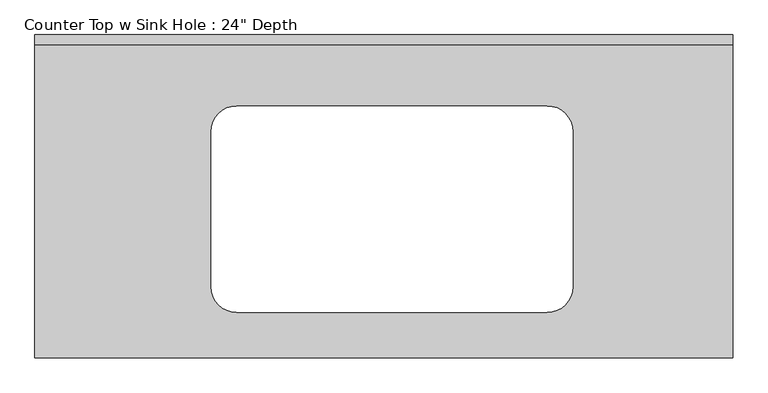
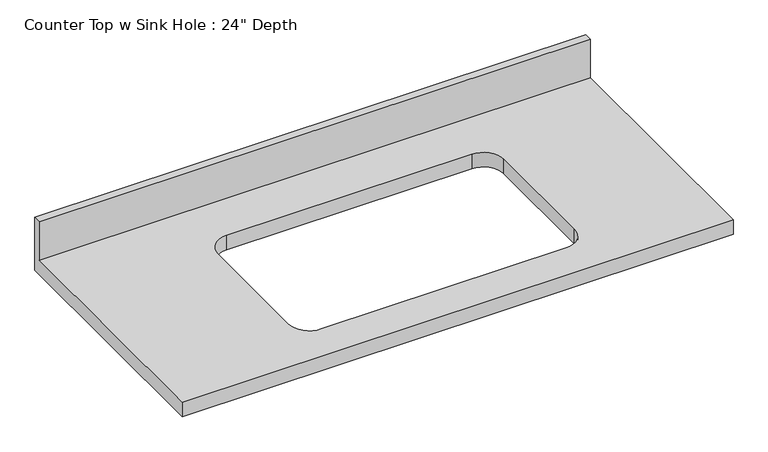
"""IFC4 building model written with IfcOpenShell, lengths in millimetres: furniture geometry."""

from ifc_helpers import new_model, si_unit, frame, origin, place, context, project, spatial, polyline, circle_curve, source, transform, mapped, element, save
from ifc_brep_helpers import plane_surface, revolved_surface, advanced_brep


def furniture_015143fb(model_context):
    return source(origin(), model_context, "Body", "AdvancedBrep", [
        advanced_brep(
        [(-1200.4622951, -635.0, 914.4), (171.1377049, -635.0, 914.4), (171.1377049, -19.05, 914.4), (-1200.4622951, -19.05, 914.4), (-803.4993371, -139.7, 914.4), (-193.8993371, -139.7, 914.4), (-143.0993371, -190.5, 914.4), (-143.0993371, -495.3, 914.4), (-193.8993371, -546.1, 914.4), (-803.4993371, -546.1, 914.4), (-854.2993371, -495.3, 914.4), (-854.2993371, -190.5, 914.4), (171.1377049, 0.0, 876.3), (171.1377049, -635.0, 876.3), (-1200.4622951, -635.0, 876.3), (-1200.4622951, 0.0, 876.3), (-193.8993371, -139.7, 876.3), (-803.4993371, -139.7, 876.3), (-854.2993371, -190.5, 876.3), (-854.2993371, -495.3, 876.3), (-803.4993371, -546.1, 876.3), (-193.8993371, -546.1, 876.3), (-143.0993371, -495.3, 876.3), (-143.0993371, -190.5, 876.3), (-1200.4622951, 0.0, 1016.0), (171.1377049, 0.0, 1016.0), (-1200.4622951, -19.05, 1016.0), (171.1377049, -19.05, 1016.0)],
        [
            (0, 1),
            (1, 2),
            (2, 3),
            (3, 0),
            (4, 5),
            (5, 6, circle_curve(frame((-193.8993371, -190.5, 914.4), z_axis=(0.0, 0.0, -1.0), x_axis=(1.0, 0.0, 0.0)), 50.8)),
            (6, 7),
            (7, 8, circle_curve(frame((-193.8993371, -495.3, 914.4), z_axis=(0.0, 0.0, -1.0), x_axis=(1.0, 0.0, 0.0)), 50.8)),
            (8, 9),
            (9, 10, circle_curve(frame((-803.4993371, -495.3, 914.4), z_axis=(0.0, 0.0, -1.0), x_axis=(1.0, 0.0, 0.0)), 50.8)),
            (10, 11),
            (11, 4, circle_curve(frame((-803.4993371, -190.5, 914.4), z_axis=(0.0, 0.0, -1.0), x_axis=(1.0, 0.0, 0.0)), 50.8)),
            (12, 13),
            (13, 14),
            (14, 15),
            (15, 12),
            (16, 17),
            (17, 18, circle_curve(frame((-803.4993371, -190.5, 876.3), z_axis=(0.0, 0.0, 1.0), x_axis=(1.0, 0.0, 0.0)), 50.8)),
            (18, 19),
            (19, 20, circle_curve(frame((-803.4993371, -495.3, 876.3), z_axis=(0.0, 0.0, 1.0), x_axis=(1.0, 0.0, 0.0)), 50.8)),
            (20, 21),
            (21, 22, circle_curve(frame((-193.8993371, -495.3, 876.3), z_axis=(0.0, 0.0, 1.0), x_axis=(1.0, 0.0, 0.0)), 50.8)),
            (22, 23),
            (23, 16, circle_curve(frame((-193.8993371, -190.5, 876.3), z_axis=(0.0, 0.0, 1.0), x_axis=(1.0, 0.0, 0.0)), 50.8)),
            (15, 24),
            (24, 25),
            (25, 12),
            (14, 0),
            (3, 26),
            (26, 24),
            (13, 1),
            (25, 27),
            (27, 2),
            (26, 27),
            (4, 17),
            (16, 5),
            (11, 18),
            (10, 19),
            (9, 20),
            (8, 21),
            (7, 22),
            (6, 23),
        ],
        [
            plane_surface(frame((-1200.4622951, 0.0, 914.4), z_axis=(0.0, 0.0, 1.0), x_axis=(-1.0, 0.0, 0.0))),
            plane_surface(frame((-1200.4622951, 0.0, 876.3), z_axis=(0.0, 0.0, -1.0), x_axis=(1.0, 0.0, 0.0))),
            plane_surface(frame((171.1377049, 0.0, 914.4), z_axis=(0.0, 1.0, 0.0), x_axis=(0.0, 0.0, -1.0))),
            plane_surface(frame((-1200.4622951, 0.0, 914.4), z_axis=(-1.0, 0.0, 0.0), x_axis=(0.0, 0.0, -1.0))),
            plane_surface(frame((-1200.4622951, -635.0, 914.4), z_axis=(0.0, -1.0, 0.0), x_axis=(0.0, 0.0, -1.0))),
            plane_surface(frame((171.1377049, -635.0, 914.4), z_axis=(1.0, 0.0, 0.0), x_axis=(0.0, 0.0, -1.0))),
            plane_surface(frame((-1200.4622951, 0.0, 1016.0), z_axis=(0.0, 0.0, 1.0), x_axis=(0.0, -1.0, 0.0))),
            plane_surface(frame((-1200.4622951, -19.05, 1016.0), z_axis=(0.0, -1.0, 0.0), x_axis=(0.0, 0.0, -1.0))),
            plane_surface(frame((-193.8993371, -139.7, 914.4), z_axis=(0.0, -1.0, 0.0), x_axis=(0.0, 0.0, -1.0))),
            revolved_surface(polyline([(-752.6993371000001, -190.5, 914.4), (-752.6993371000001, -190.5, 876.3)]), (-803.4993371, -190.5, 876.3), (0.0, 0.0, 1.0)),
            plane_surface(frame((-854.2993371, -190.5, 914.4), z_axis=(1.0, 0.0, 0.0), x_axis=(0.0, 0.0, -1.0))),
            revolved_surface(polyline([(-752.6993371000001, -495.3, 914.4), (-752.6993371000001, -495.3, 876.3)]), (-803.4993371, -495.3, 876.3), (0.0, 0.0, 1.0)),
            plane_surface(frame((-803.4993371, -546.1, 914.4), z_axis=(0.0, 1.0, 0.0), x_axis=(0.0, 0.0, -1.0))),
            revolved_surface(polyline([(-143.0993371, -495.3, 914.4), (-143.0993371, -495.3, 876.3)]), (-193.8993371, -495.3, 876.3), (0.0, 0.0, 1.0)),
            plane_surface(frame((-143.0993371, -495.3, 914.4), z_axis=(-1.0, 0.0, 0.0), x_axis=(0.0, 0.0, -1.0))),
            revolved_surface(polyline([(-143.0993371, -190.5, 914.4), (-143.0993371, -190.5, 876.3)]), (-193.8993371, -190.5, 876.3), (0.0, 0.0, 1.0)),
        ],
        [
            (0, [[1, 2, 3, 4], [5, 6, 7, 8, 9, 10, 11, 12]]),
            (1, [[13, 14, 15, 16], [17, 18, 19, 20, 21, 22, 23, 24]]),
            (2, [[-16, 25, 26, 27]]),
            (3, [[-15, 28, -4, 29, 30, -25]]),
            (4, [[-1, -28, -14, 31]]),
            (5, [[-13, -27, 32, 33, -2, -31]]),
            (6, [[-30, 34, -32, -26]]),
            (7, [[-34, -29, -3, -33]]),
            (8, [[35, -17, 36, -5]]),
            (9, [[-35, -12, 37, -18]]),
            (10, [[-37, -11, 38, -19]]),
            (11, [[-38, -10, 39, -20]]),
            (12, [[-39, -9, 40, -21]]),
            (13, [[-40, -8, 41, -22]]),
            (14, [[-41, -7, 42, -23]]),
            (15, [[-36, -24, -42, -6]]),
        ],
    ),
    ])


if __name__ == "__main__":
    model = new_model("IFC4")
    model_context = context("Model", 3, world=origin())
    ifc_project = project(units=[si_unit("LENGTHUNIT", "METRE", prefix="MILLI")], contexts=[model_context])
    site = spatial("IfcSite", under=ifc_project)
    building = spatial("IfcBuilding", under=site)
    placement = place(None, origin())
    furniture_shape = furniture_015143fb(model_context)
    element("IfcFurniture", 1, ObjectType="Counter Top w Sink Hole : 24\" Depth", at=placement, inside=building, context=model_context, shape_type="MappedRepresentation", body=[
        mapped(furniture_shape, transform((0.0, 0.0, 0.0), x_axis=(1.0, 0.0, 0.0), y_axis=(0.0, 1.0, 0.0), z_axis=(0.0, 0.0, 1.0))),
    ])
    save(model, "model.ifc")

# Revit data of these elements
# Type "Counter Top w Sink Hole : 24\" Depth"
#   Assembly Code = "C1030400"
#   Counter Thickness = 0' - 1 1/2"
#   Depth = 2' - 1"
#   Height = 3' - 0"
#   Length [instance default] = 8' - 0"
#   Sink Location [instance default] = 2' - 0"
#   Sink Location To Wall [instance default] = 0' - 6"
#   Sink Opening Depth [instance default] = 1' - 3"
#   Sink Opening Width [instance default] = 2' - 3"
#   Counter Top Material = none
#   Default Elevation = 0
# Element 1 (IfcFurniture, "Counter Top w Sink Hole : 24\" Depth")
#   Length = 4' - 6"
#   Sink Location = 2' - 3.62846"
#   Materials on its faces: "Counter Top"
# Materials
#   "Counter Top": class "Wood", colour RGB 226 177 128, transparency 0
